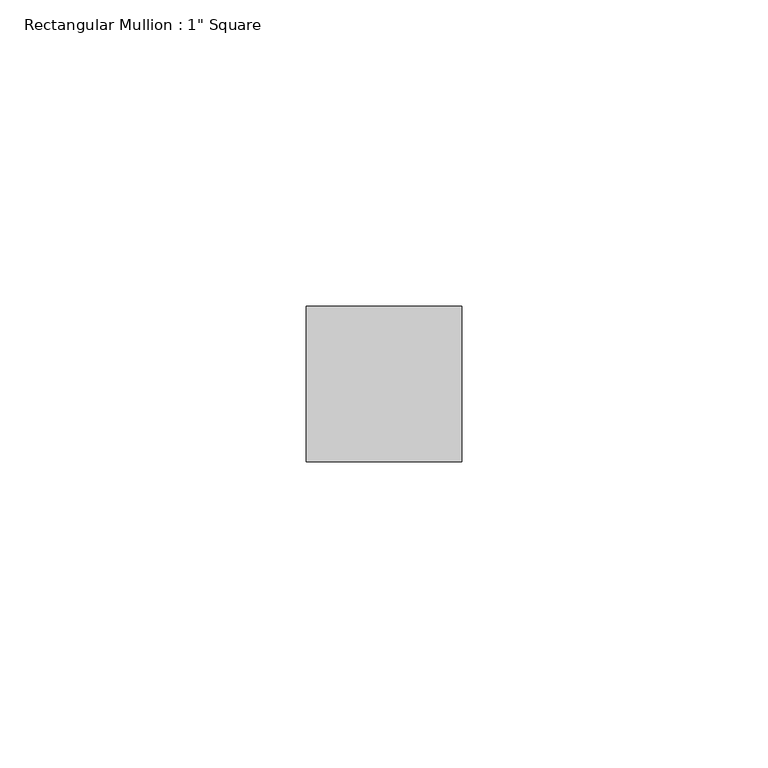
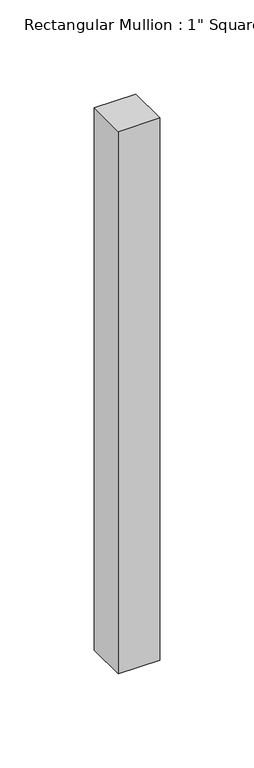
"""IFC4 building model written with IfcOpenShell, lengths in millimetres: member geometry."""

from ifc_helpers import new_model, si_unit, frame, origin, place, context, project, spatial, polyline, outline, extrude, source, transform, mapped, element, save


def member_2ec808cb(model_context):
    return source(origin(), model_context, "Body", "SweptSolid", [
        extrude(outline(polyline([(12.7, 12.7), (12.7, -12.7), (-12.7, -12.7), (-12.7, 12.7), (12.7, 12.7)])), frame((0.0, 0.0, -351.3666667), z_axis=(0.0, 0.0, 1.0), x_axis=(1.0, 0.0, 0.0)), (0.0, 0.0, 1.0), 351.3666667),
    ])


if __name__ == "__main__":
    model = new_model("IFC4")
    model_context = context("Model", 3, world=origin())
    ifc_project = project(units=[si_unit("LENGTHUNIT", "METRE", prefix="MILLI")], contexts=[model_context])
    site = spatial("IfcSite", under=ifc_project)
    building = spatial("IfcBuilding", under=site)
    placement = place(None, origin())
    member_shape = member_2ec808cb(model_context)
    element("IfcMember", 1, ObjectType="Rectangular Mullion : 1\" Square", at=placement, inside=building, context=model_context, shape_type="MappedRepresentation", body=[
        mapped(member_shape, transform((0.0, 0.0, 0.0), x_axis=(1.0, 0.0, 0.0), y_axis=(0.0, 1.0, 0.0), z_axis=(0.0, 0.0, 1.0))),
    ])
    save(model, "model.ifc")

# Revit data of these elements
# Type "Rectangular Mullion : 1\" Square"
#   built-in parameter 1007304 = 0.0833333 (stored number, unit not read)
#   built-in parameter 1007301 = 0.0416667 (stored number, unit not read)
#   built-in parameter 1007300 = 0.0416667 (stored number, unit not read)
# Element 1 (IfcMember, "Rectangular Mullion : 1\" Square")
#   Materials on its faces: "Aluminum"
# Materials
#   "Aluminum": class "Metal", colour RGB 247 247 247, transparency 0, Description = "Aluminum 6061", Cost = 0
